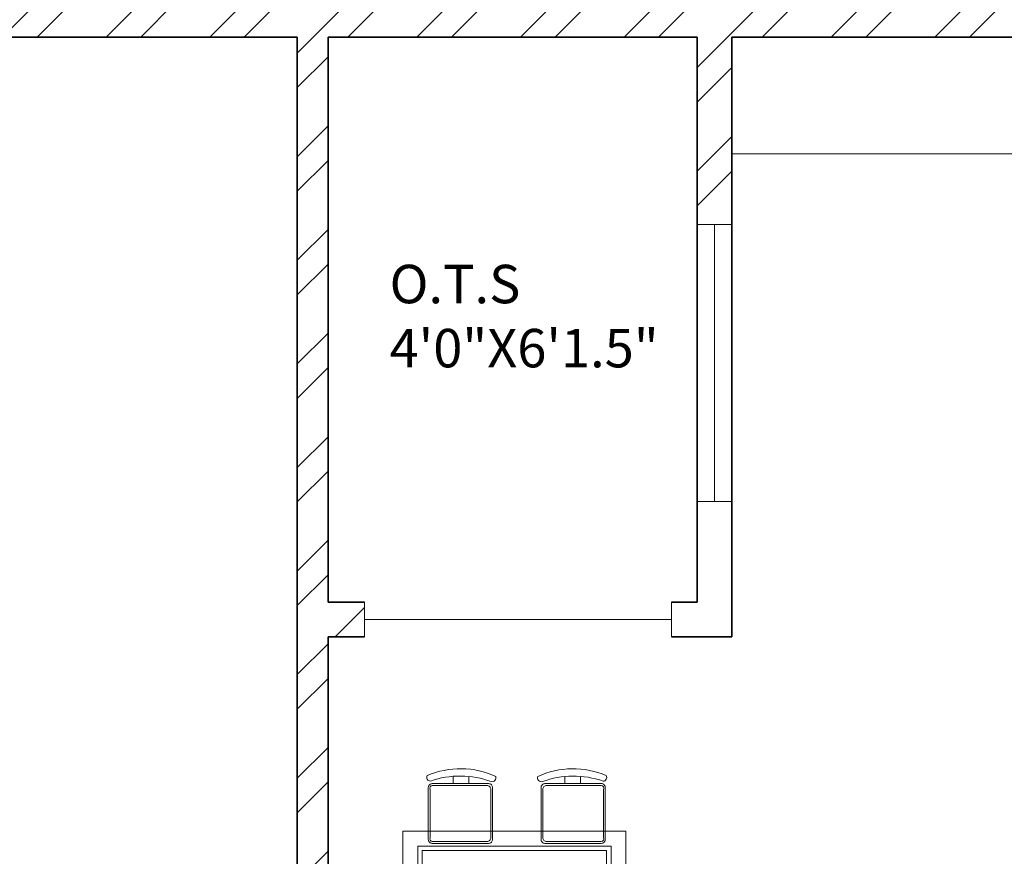
# Model space of a CAD drawing. Units: inches. Extents: x 2120 to 4013, y 1390 to 3019.
# Tile 30 of 59: x 2356 to 2484, y 1964 to 2073. Entities that reach past the tile are written whole.
import ezdxf

# ---------------------------------------------------------------- set-up
doc = ezdxf.new("R2010")
doc.units = ezdxf.units.IN
for name, color, linetype, lineweight in [('A-AREA-IDEN', 7, 'Continuous', 18), ('A-FLOR-CASE', 8, 'Continuous', 18), ('A-FURN', 8, 'Continuous', 13), ('A-GLAZ', 4, 'Continuous', 18), ('A-WALL', 7, 'Continuous', 35), ('A-WALL-PATT', 252, 'Continuous', 13)]:
    doc.layers.add(name, color=color, linetype=linetype, lineweight=lineweight)
doc.styles.get("Standard").update_dxf_attribs({"font": 'arial.ttf'})

# ---------------------------------------------------------------- blocks, each defined once
blk = doc.blocks.new('WIN-PLAN-36IN-02')
for p, q in [((2.25, 36), (0, 36)), ((0, 36), (4.5, 36)), ((2.25, 0), (2.25, 36)), ((0, 0), (4.5, 0)), ((4.5, 0), (2.25, 0))]:
    blk.add_line(p, q)
blk = doc.blocks.new('WIN-PLAN-40IN')
for p, q in [((0, 4.5), (0, 0)), ((39.95, 4.5), (39.95, 0)), ((39.95, 2.25), (0, 2.25)), ((39.95, 0), (39.95, 2.25))]:
    blk.add_line(p, q)
blk = doc.blocks.new('TABLE-DINING')
for points in [[(0, 17.41), (29.01, 17.41), (29.01, 0), (0, 0)], [(1.93, 15.47), (27.08, 15.47), (27.08, 1.93), (1.93, 1.93)], [(2.51, 14.89), (26.5, 14.89), (26.5, 2.51), (2.51, 2.51)]]:
    blk.add_lwpolyline(points, close=True)
blk = doc.blocks.new('CHAIR-DINING-01')
for points in [[(1.68, 0.62, -0.578392), (1.02, 0.02, -0.214524), (0.9, 8.94, -0.552014), (1.62, 8.52, 0.175809), (1.68, 0.62)], [(1.93, 8.29, -0.414214), (2.45, 8.81), (9.19, 8.81, -0.414214), (9.7, 8.29), (9.7, 0.96, -0.414214), (9.19, 0.45), (2.45, 0.45, -0.414214), (1.93, 0.96), (1.93, 8.29)], [(1.93, 3.54), (1.01, 3.54, 0.064759)]]:
    blk.add_lwpolyline(points, format="xyb")
blk.add_lwpolyline([(2.16, 8.29), (2.16, 1.19, 0.414214), (2.68, 0.68), (8.96, 0.68, 0.414214), (9.47, 1.19), (9.47, 8.29, 0.512069), (8.96, 8.58), (2.68, 8.58, 0.512069)], format="xyb", close=True)
blk.add_lwpolyline([(0.99, 5.59), (1.93, 5.59)])
blk = doc.blocks.new('CHAIR-DINING-05')
for points in [[(1.68, 0.62, -0.578392), (1.02, 0.02, -0.214524), (0.9, 8.94, -0.552014), (1.62, 8.52, 0.175809), (1.68, 0.62)], [(1.93, 8.29, -0.414214), (2.45, 8.81), (9.19, 8.81, -0.414214), (9.7, 8.29), (9.7, 0.96, -0.414214), (9.19, 0.45), (2.45, 0.45, -0.414214), (1.93, 0.96), (1.93, 8.29)], [(1.93, 3.54), (1.01, 3.54, 0.064759)]]:
    blk.add_lwpolyline(points, format="xyb")
blk.add_lwpolyline([(2.16, 8.29), (2.16, 1.19, 0.414214), (2.68, 0.68), (8.96, 0.68, 0.414214), (9.47, 1.19), (9.47, 8.29, 0.512069), (8.96, 8.58), (2.68, 8.58, 0.512069)], format="xyb", close=True)
blk.add_lwpolyline([(0.99, 5.59), (1.93, 5.59)])
blk = doc.blocks.new('CHAIR-DINING-08')
for points in [[(0.47, 8.09, -0.175809), (8.38, 8.03, 0.578392), (8.97, 8.69, 0.214524), (0.06, 8.81, 0.552014), (0.47, 8.09, -0.065079)], [(8.04, 7.77), (0.71, 7.77, 0.414214), (0.19, 7.26), (0.19, 0.51, 0.414214), (0.71, 0), (8.04, 0, 0.414214), (8.55, 0.51), (8.55, 7.26, 0.414214), (8.04, 7.77)], [(5.46, 7.77), (5.46, 8.7, -0.064759)]]:
    blk.add_lwpolyline(points, format="xyb")
blk.add_lwpolyline([(3.41, 8.72), (3.41, 7.77)])
blk.add_lwpolyline([(0.71, 7.54), (7.81, 7.54, -0.414214), (8.32, 7.03), (8.32, 0.74, -0.414214), (7.81, 0.23), (0.71, 0.23, -0.512069), (0.42, 0.74), (0.42, 7.03, -0.512069)], format="xyb", close=True)
blk = doc.blocks.new('CHAIR-DINING-13')
for points in [[(0.47, 8.09, -0.175809), (8.38, 8.03, 0.578392), (8.97, 8.69, 0.214524), (0.06, 8.81, 0.552014), (0.47, 8.09, -0.065079)], [(8.04, 7.77), (0.71, 7.77, 0.414214), (0.19, 7.26), (0.19, 0.51, 0.414214), (0.71, 0), (8.04, 0, 0.414214), (8.55, 0.51), (8.55, 7.26, 0.414214), (8.04, 7.77)], [(5.46, 7.77), (5.46, 8.7, -0.064759)]]:
    blk.add_lwpolyline(points, format="xyb")
blk.add_lwpolyline([(3.41, 8.72), (3.41, 7.77)])
blk.add_lwpolyline([(0.71, 7.54), (7.81, 7.54, -0.414214), (8.32, 7.03), (8.32, 0.74, -0.414214), (7.81, 0.23), (0.71, 0.23, -0.512069), (0.42, 0.74), (0.42, 7.03, -0.512069)], format="xyb", close=True)

msp = doc.modelspace()

# ---------------------------------------------------------------- hatches: boundary and pattern name
at = {"layer": 'A-WALL-PATT'}
h = msp.add_hatch(dxfattribs=at)
h.set_pattern_fill('ANSI32', color=256)
h.paths.add_polyline_path([(2271.7331, 2343.531), (2283.3788, 2343.531), (2283.3788, 2348.031), (2283.3788, 2352.5306), (2262.7331, 2352.5306), (2262.7331, 2182.638), (2267.2331, 2182.638), (2271.7331, 2182.638), (2271.7331, 2219.031), (2391.7331, 2219.031), (2391.7331, 2214.189), (2393.9831, 2214.189), (2396.2331, 2214.189), (2396.2331, 2219.031), (2420.2331, 2219.031), (2420.2331, 2225.7535), (2417.2197, 2225.7535), (2415.7331, 2225.7535), (2415.7331, 2223.5306), (2271.7331, 2223.5306)])
h.paths.add_polyline_path([(2380.0942, 2352.5306), (2343.3788, 2352.5306), (2343.3788, 2343.531), (2363.2331, 2343.531), (2363.2331, 2288.8489), (2365.4831, 2288.8489), (2367.7331, 2288.8489), (2367.7331, 2343.531), (2380.0942, 2343.531)], flags=17)
h.paths.add_polyline_path([(2432.4339, 2352.5306), (2404.0943, 2352.5306), (2404.0943, 2343.531), (2415.7331, 2343.531), (2415.7331, 2264.0306), (2367.7331, 2264.0306), (2367.7331, 2266.4872), (2363.2331, 2266.4872), (2363.2331, 2259.531), (2367.7331, 2259.531), (2415.7331, 2259.531), (2415.7331, 2255.0658), (2420.2331, 2255.0658), (2420.2331, 2259.531), (2424.5717, 2259.531), (2424.5717, 2261.781), (2424.5717, 2264.0306), (2420.2331, 2264.0306), (2420.2331, 2343.531), (2432.4339, 2343.531)])
h.paths.add_polyline_path([(2508.9115, 2352.5306), (2456.4339, 2352.5306), (2456.4339, 2343.531), (2468.2331, 2343.531), (2468.2331, 2264.0306), (2448.0487, 2264.0306), (2448.0487, 2259.531), (2468.2331, 2259.531), (2468.2331, 2255.5496), (2472.7331, 2255.5496), (2472.7331, 2343.531), (2508.9115, 2343.531)])
h.paths.add_polyline_path([(2637.7331, 2352.5306), (2544.9116, 2352.5306), (2544.9116, 2343.531), (2589.7331, 2343.531), (2633.2331, 2343.531), (2637.7331, 2343.531)])
h.paths.add_polyline_path([(2594.2331, 2343.5306), (2589.7331, 2343.5306), (2589.7331, 2259.5306), (2589.7331, 2252.4915), (2591.9831, 2252.4915), (2594.2331, 2252.4915)])
h.paths.add_polyline_path([(2637.7331, 2223.5306), (2594.2331, 2223.5306), (2594.2331, 2230.1988), (2591.9831, 2230.1988), (2589.7331, 2230.1988), (2589.7331, 2223.5306), (2472.7331, 2223.5306), (2468.2331, 2223.5306), (2468.2331, 2219.031), (2628.7331, 2219.031), (2628.7331, 2138.031), (2637.7331, 2138.031)])
h.paths.add_polyline_path([(3822.6535, 2458.4402), (3874.9468, 2458.4402), (3874.9468, 2476.9866), (3822.6535, 2476.9866)], flags=9)
h.paths.add_polyline_path([(3834.6921, 2781.8174), (3935.9206, 2781.8174), (3935.9206, 2800.3638), (3834.6921, 2800.3638)], flags=9)
h.paths.add_polyline_path([(3832.2843, 2837.9683), (3884.5776, 2837.9683), (3884.5776, 2856.5146), (3832.2843, 2856.5146)], flags=9)
h.paths.add_polyline_path([(3830.9388, 2861.4782), (3956.8958, 2861.4782), (3956.8958, 2880.0245), (3830.9388, 2880.0245)], flags=9)
h.paths.add_polyline_path([(3870.6966, 2352.5752), (3887.9272, 2352.5752), (3887.9272, 2377.3037), (3870.6966, 2377.3037)], flags=9)
h.paths.add_polyline_path([(3289.2701, 2413.161), (3435.2223, 2413.161), (3435.2223, 2450.2538), (3289.2701, 2450.2538)], flags=9)
h.paths.add_polyline_path([(2487.6944, 2414.3601), (2637.8335, 2414.3601), (2637.8335, 2451.4528), (2487.6944, 2451.4528)], flags=9)
h.paths.add_polyline_path([(2567.3724, 1457.9199), (2815.296, 1457.9199), (2815.296, 1495.0127), (2567.3724, 1495.0127)], flags=9)
h.paths.add_polyline_path([(2655.3825, 2093.2363), (2685.9555, 2093.2363), (2685.9555, 2111.8937), (2655.3825, 2111.8937)], flags=9)
h.paths.add_polyline_path([(2543.9218, 1550.6671), (2587.8406, 1550.6671), (2587.8406, 1569.3244), (2543.9218, 1569.3244)], flags=9)
h.paths.add_polyline_path([(2905.1384, 1543.8113), (2949.0572, 1543.8113), (2949.0572, 1562.4686), (2905.1384, 1562.4686)], flags=9)
h.paths.add_polyline_path([(2736.4118, 1702.4736), (2784.2153, 1702.4736), (2784.2153, 1721.1309), (2736.4118, 1721.1309)], flags=9)
h.paths.add_polyline_path([(2912.8666, 1710.4168), (2951.707, 1710.4168), (2951.707, 1729.0741), (2912.8666, 1729.0741)], flags=9)
h.paths.add_polyline_path([(2923.5785, 1763.5038), (2959.7279, 1763.5038), (2959.7279, 1782.1611), (2923.5785, 1782.1611)], flags=9)
h.paths.add_polyline_path([(2925.2114, 1809.6137), (2967.1861, 1809.6137), (2967.1861, 1828.271), (2925.2114, 1828.271)], flags=9)
h.paths.add_polyline_path([(2996.2711, 1878.9003), (2996.2711, 1913.109), (2977.6138, 1913.109), (2977.6138, 1878.9003)], flags=9)
h.paths.add_polyline_path([(2883.0859, 1895.7192), (2927.1855, 1895.7192), (2927.1855, 1914.3766), (2883.0859, 1914.3766)], flags=9)
h.paths.add_polyline_path([(2787.3924, 1810.8013), (2841.0213, 1810.8013), (2841.0213, 1829.4587), (2787.3924, 1829.4587)], flags=9)
h.paths.add_polyline_path([(2775.6399, 2101.7395), (2829.2689, 2101.7395), (2829.2689, 2120.3968), (2775.6399, 2120.3968)], flags=9)
h.paths.add_polyline_path([(2913.0263, 2075.817), (2951.8667, 2075.817), (2951.8667, 2094.4744), (2913.0263, 2094.4744)], flags=9)
h.paths.add_polyline_path([(2929.966, 2133.3669), (2966.1154, 2133.3669), (2966.1154, 2152.0243), (2929.966, 2152.0243)], flags=9)
h.paths.add_polyline_path([(2932.7502, 2182.6088), (2968.8996, 2182.6088), (2968.8996, 2201.2662), (2932.7502, 2201.2662)], flags=9)
h.paths.add_polyline_path([(2996.0681, 2266.3173), (2996.0681, 2300.5261), (2977.4108, 2300.5261), (2977.4108, 2266.3173)], flags=9)
h.paths.add_polyline_path([(2885.1039, 2279.2186), (2929.2035, 2279.2186), (2929.2035, 2297.8759), (2885.1039, 2297.8759)], flags=9)
h.paths.add_polyline_path([(2735.7042, 2218.3197), (2783.5078, 2218.3197), (2783.5078, 2236.9771), (2735.7042, 2236.9771)], flags=9)
h.paths.add_polyline_path([(2635.6049, 2044.0085), (2648.9678, 2044.0085), (2648.9678, 2054.312), (2635.6049, 2054.312)], flags=9)
h.paths.add_polyline_path([(2714.0148, 1923.0473), (2727.3777, 1923.0473), (2727.3777, 1933.3508), (2714.0148, 1933.3508)], flags=9)
h.paths.add_polyline_path([(2709.0345, 1988.1628), (2722.3974, 1988.1628), (2722.3974, 1998.4663), (2709.0345, 1998.4663)], flags=9)
h.paths.add_polyline_path([(2592.8935, 1962.1763), (2606.2564, 1962.1763), (2606.2564, 1972.4799), (2592.8935, 1972.4799)], flags=9)
h.paths.add_polyline_path([(2618.3996, 1985.9724), (2644.1942, 1985.9724), (2644.1942, 1996.2759), (2618.3996, 1996.2759)], flags=9)
h.paths.add_polyline_path([(2601.279, 1920.5869), (2614.6419, 1920.5869), (2614.6419, 1930.8904), (2601.279, 1930.8904)], flags=9)
h.paths.add_polyline_path([(2692.3278, 1932.7645), (2704.5311, 1932.7645), (2704.5311, 1943.0681), (2692.3278, 1943.0681)], flags=9)
h.paths.add_polyline_path([(2311.122, 1672.7318), (2355.0408, 1672.7318), (2355.0408, 1691.3892), (2311.122, 1691.3892)], flags=9)
h.paths.add_polyline_path([(2456.2551, 1632.3198), (2492.4796, 1632.3198), (2492.4796, 1650.9772), (2456.2551, 1650.9772)], flags=9)
h.paths.add_polyline_path([(2401.0766, 1631.4793), (2437.301, 1631.4793), (2437.301, 1650.1367), (2401.0766, 1650.1367)], flags=9)
h.paths.add_polyline_path([(2546.7054, 1700.9235), (2594.509, 1700.9235), (2594.509, 1719.5809), (2546.7054, 1719.5809)], flags=9)
h.paths.add_polyline_path([(2445.4866, 1766.9937), (2497.5261, 1766.9937), (2497.5261, 1785.651), (2445.4866, 1785.651)], flags=9)
h.paths.add_polyline_path([(2287.9992, 1739.7675), (2326.8396, 1739.7675), (2326.8396, 1758.4248), (2287.9992, 1758.4248)], flags=9)
h.paths.add_polyline_path([(2458.5279, 1924.7607), (2510.5675, 1924.7607), (2510.5675, 1943.4181), (2458.5279, 1943.4181)], flags=9)
h.paths.add_polyline_path([(2309.2811, 1902.7642), (2345.4305, 1902.7642), (2345.4305, 1921.4215), (2309.2811, 1921.4215)], flags=9)
h.paths.add_polyline_path([(2490.7554, 2018.9392), (2530.7896, 2018.9392), (2530.7896, 2037.5965), (2490.7554, 2037.5965)], flags=9)
h.paths.add_polyline_path([(2402.143, 2024.7393), (2438.5414, 2024.7393), (2438.5414, 2043.3966), (2402.143, 2043.3966)], flags=9)
h.paths.add_polyline_path([(2287.856, 1931.7926), (2326.6964, 1931.7926), (2326.6964, 1950.4499), (2287.856, 1950.4499)], flags=9)
h.paths.add_polyline_path([(2281.7979, 2193.5771), (2320.6383, 2193.5771), (2320.6383, 2212.2344), (2281.7979, 2212.2344)], flags=25)
h.paths.add_polyline_path([(2484.0754, 2093.892), (2536.115, 2093.892), (2536.115, 2112.5494), (2484.0754, 2112.5494)], flags=9)
h.paths.add_polyline_path([(2624.7948, 2281.8639), (2624.7948, 2311.4137), (2606.1375, 2311.4137), (2606.1375, 2281.8639)], flags=9)
h.paths.add_polyline_path([(2507.5036, 2290.3639), (2541.934, 2290.3639), (2541.934, 2309.0212), (2507.5036, 2309.0212)], flags=9)
h.paths.add_polyline_path([(2423.1076, 2285.2202), (2459.332, 2285.2202), (2459.332, 2303.8776), (2423.1076, 2303.8776)], flags=9)
h.paths.add_polyline_path([(2374.5467, 2289.6272), (2410.7711, 2289.6272), (2410.7711, 2308.2846), (2374.5467, 2308.2846)], flags=25)
h.paths.add_polyline_path([(2277.4907, 2227.5651), (2316.3311, 2227.5651), (2316.3311, 2246.2224), (2277.4907, 2246.2224)], flags=25)
h.paths.add_polyline_path([(2655.3825, 2093.2367), (2685.9555, 2093.2367), (2685.9555, 2111.894), (2655.3825, 2111.894)], flags=9)
h.paths.add_polyline_path([(2543.9217, 1550.6674), (2587.8406, 1550.6674), (2587.8406, 1569.3247), (2543.9217, 1569.3247)], flags=9)
h.paths.add_polyline_path([(2905.1384, 1543.8116), (2949.0572, 1543.8116), (2949.0572, 1562.4689), (2905.1384, 1562.4689)], flags=9)
h.paths.add_polyline_path([(2736.4118, 1702.4739), (2784.2153, 1702.4739), (2784.2153, 1721.1312), (2736.4118, 1721.1312)], flags=9)
h.paths.add_polyline_path([(2912.8666, 1710.4171), (2951.707, 1710.4171), (2951.707, 1729.0744), (2912.8666, 1729.0744)], flags=9)
h.paths.add_polyline_path([(2923.5785, 1763.5041), (2959.7279, 1763.5041), (2959.7279, 1782.1614), (2923.5785, 1782.1614)], flags=9)
h.paths.add_polyline_path([(2925.2114, 1809.614), (2967.1861, 1809.614), (2967.1861, 1828.2713), (2925.2114, 1828.2713)], flags=9)
h.paths.add_polyline_path([(2996.2711, 1878.9006), (2996.2711, 1913.1094), (2977.6137, 1913.1094), (2977.6137, 1878.9006)], flags=9)
h.paths.add_polyline_path([(2883.0859, 1895.7195), (2927.1855, 1895.7195), (2927.1855, 1914.3769), (2883.0859, 1914.3769)], flags=9)
h.paths.add_polyline_path([(2787.3924, 1810.8016), (2841.0213, 1810.8016), (2841.0213, 1829.459), (2787.3924, 1829.459)], flags=9)
h.paths.add_polyline_path([(2775.6399, 2101.7398), (2829.2688, 2101.7398), (2829.2688, 2120.3971), (2775.6399, 2120.3971)], flags=9)
h.paths.add_polyline_path([(2913.0263, 2075.8173), (2951.8667, 2075.8173), (2951.8667, 2094.4747), (2913.0263, 2094.4747)], flags=9)
h.paths.add_polyline_path([(2929.966, 2133.3672), (2966.1154, 2133.3672), (2966.1154, 2152.0246), (2929.966, 2152.0246)], flags=9)
h.paths.add_polyline_path([(2932.7502, 2182.6091), (2968.8996, 2182.6091), (2968.8996, 2201.2665), (2932.7502, 2201.2665)], flags=9)
h.paths.add_polyline_path([(2996.0681, 2266.3176), (2996.0681, 2300.5264), (2977.4108, 2300.5264), (2977.4108, 2266.3176)], flags=9)
h.paths.add_polyline_path([(2885.1039, 2279.2189), (2929.2035, 2279.2189), (2929.2035, 2297.8762), (2885.1039, 2297.8762)], flags=9)
h.paths.add_polyline_path([(2735.7042, 2218.32), (2783.5078, 2218.32), (2783.5078, 2236.9774), (2735.7042, 2236.9774)], flags=9)
h.paths.add_polyline_path([(2635.6048, 2044.0088), (2648.9677, 2044.0088), (2648.9677, 2054.3123), (2635.6048, 2054.3123)], flags=9)
h.paths.add_polyline_path([(2714.0148, 1923.0476), (2727.3777, 1923.0476), (2727.3777, 1933.3511), (2714.0148, 1933.3511)], flags=9)
h.paths.add_polyline_path([(2709.0345, 1988.1631), (2722.3974, 1988.1631), (2722.3974, 1998.4666), (2709.0345, 1998.4666)], flags=9)
h.paths.add_polyline_path([(2592.8935, 1962.1766), (2606.2564, 1962.1766), (2606.2564, 1972.4802), (2592.8935, 1972.4802)], flags=9)
h.paths.add_polyline_path([(2618.3995, 1985.9727), (2644.1942, 1985.9727), (2644.1942, 1996.2762), (2618.3995, 1996.2762)], flags=9)
h.paths.add_polyline_path([(2601.279, 1920.5872), (2614.6419, 1920.5872), (2614.6419, 1930.8908), (2601.279, 1930.8908)], flags=9)
h.paths.add_polyline_path([(2692.3278, 1932.7648), (2704.5311, 1932.7648), (2704.5311, 1943.0684), (2692.3278, 1943.0684)], flags=9)
h.paths.add_polyline_path([(2311.122, 1672.7321), (2355.0408, 1672.7321), (2355.0408, 1691.3895), (2311.122, 1691.3895)], flags=9)
h.paths.add_polyline_path([(2456.2551, 1632.3201), (2492.4795, 1632.3201), (2492.4795, 1650.9775), (2456.2551, 1650.9775)], flags=9)
h.paths.add_polyline_path([(2401.0766, 1631.4796), (2437.301, 1631.4796), (2437.301, 1650.137), (2401.0766, 1650.137)], flags=9)
h.paths.add_polyline_path([(2546.7054, 1700.9238), (2594.509, 1700.9238), (2594.509, 1719.5812), (2546.7054, 1719.5812)], flags=9)
h.paths.add_polyline_path([(2445.4866, 1766.994), (2497.5261, 1766.994), (2497.5261, 1785.6513), (2445.4866, 1785.6513)], flags=9)
h.paths.add_polyline_path([(2287.9992, 1739.7678), (2326.8396, 1739.7678), (2326.8396, 1758.4251), (2287.9992, 1758.4251)], flags=9)
h.paths.add_polyline_path([(2458.5279, 1924.7611), (2510.5675, 1924.7611), (2510.5675, 1943.4184), (2458.5279, 1943.4184)], flags=9)
h.paths.add_polyline_path([(2309.2811, 1902.7645), (2345.4305, 1902.7645), (2345.4305, 1921.4218), (2309.2811, 1921.4218)], flags=9)
h.paths.add_polyline_path([(2490.7554, 2018.9395), (2530.7895, 2018.9395), (2530.7895, 2037.5968), (2490.7554, 2037.5968)], flags=9)
h.paths.add_polyline_path([(2402.143, 2024.7396), (2438.5413, 2024.7396), (2438.5413, 2043.3969), (2402.143, 2043.3969)], flags=9)
h.paths.add_polyline_path([(2287.856, 1931.7929), (2326.6964, 1931.7929), (2326.6964, 1950.4502), (2287.856, 1950.4502)], flags=9)
h.paths.add_polyline_path([(2281.7979, 2193.5774), (2320.6383, 2193.5774), (2320.6383, 2212.2347), (2281.7979, 2212.2347)], flags=25)
h.paths.add_polyline_path([(2484.0754, 2093.8924), (2536.115, 2093.8924), (2536.115, 2112.5497), (2484.0754, 2112.5497)], flags=9)
h.paths.add_polyline_path([(2624.7948, 2281.8642), (2624.7948, 2311.414), (2606.1374, 2311.414), (2606.1374, 2281.8642)], flags=9)
h.paths.add_polyline_path([(2507.5035, 2290.3642), (2541.934, 2290.3642), (2541.934, 2309.0215), (2507.5035, 2309.0215)], flags=9)
h.paths.add_polyline_path([(2423.1075, 2285.2205), (2459.332, 2285.2205), (2459.332, 2303.8779), (2423.1075, 2303.8779)], flags=9)
h.paths.add_polyline_path([(2374.5467, 2289.6275), (2410.7711, 2289.6275), (2410.7711, 2308.2849), (2374.5467, 2308.2849)], flags=25)
h.paths.add_polyline_path([(2277.4907, 2227.5654), (2316.3311, 2227.5654), (2316.3311, 2246.2227), (2277.4907, 2246.2227)], flags=25)
h = msp.add_hatch(dxfattribs=at)
h.set_pattern_fill('ANSI32', color=256)
h.paths.add_polyline_path([(2271.7331, 1980.389), (2262.7331, 1980.389), (2262.7331, 1912.8434), (2267.2331, 1912.8434), (2271.7331, 1912.8434), (2271.7331, 1922.531), (2351.2331, 1922.531), (2351.2331, 1901.4728), (2355.7331, 1901.4728), (2355.7331, 1922.531), (2357.9815, 1922.531), (2357.9815, 1926.5306), (2271.7331, 1926.5306)])
h.paths.add_polyline_path([(2589.2331, 1949.1622), (2584.7331, 1949.1622), (2580.2331, 1949.1622), (2580.2331, 1874.5306), (2355.7331, 1874.5306), (2355.7331, 1880.1922), (2351.2331, 1880.1922), (2351.2331, 1874.5306), (2271.7331, 1874.5306), (2271.7331, 1888.8431), (2262.7331, 1888.8431), (2262.7331, 1842.2909), (2267.2331, 1842.2909), (2271.7331, 1842.2909), (2271.7331, 1865.531), (2415.7331, 1865.531), (2415.7331, 1779.7286), (2420.2331, 1779.7286), (2420.2331, 1865.531), (2589.2331, 1865.531)])
h.paths.add_polyline_path([(2271.7331, 1782.2906), (2262.7331, 1782.2906), (2262.7331, 1711.4639), (2267.2331, 1711.4639), (2271.7331, 1711.4639), (2271.7331, 1738.031), (2420.2331, 1738.031), (2420.2331, 1742.531), (2420.2331, 1747.3376), (2417.9831, 1747.3376), (2415.7331, 1747.3376), (2415.7331, 1742.5306), (2271.7331, 1742.5306)])
h.paths.add_polyline_path([(2271.7331, 1627.031), (2362.3957, 1627.031), (2362.3957, 1629.281), (2362.3957, 1631.5306), (2271.7331, 1631.5306), (2271.7331, 1675.4636), (2262.7331, 1675.4636), (2262.7331, 1581.531), (2405.3032, 1581.531), (2405.3032, 1586.031), (2405.3032, 1590.5306), (2396.2331, 1590.5306), (2396.2331, 1691.4513), (2418.7206, 1691.4513), (2418.7206, 1695.951), (2396.2331, 1695.951), (2391.7331, 1695.951), (2391.7331, 1631.5306), (2386.7425, 1631.5306), (2386.7425, 1629.2806), (2386.7425, 1627.031), (2391.7331, 1627.031), (2391.7331, 1586.1709), (2271.7331, 1586.1709)])
h.paths.add_polyline_path([(2459.6703, 1590.5306), (2429.3032, 1590.5306), (2429.3032, 1581.531), (2459.6703, 1581.531), (2459.6703, 1586.031)])
h.paths.add_polyline_path([(2501.2331, 1590.531), (2501.2331, 1665.0195), (2498.9831, 1665.0195), (2496.7331, 1665.0195), (2496.7331, 1590.5306), (2483.8201, 1590.5306), (2483.8201, 1590.1579), (2483.6704, 1590.1579), (2483.6704, 1581.531), (2505.0196, 1581.531), (2505.0196, 1583.781), (2505.0196, 1586.0306), (2501.2331, 1586.0306)])
h.paths.add_polyline_path([(2544.1361, 1583.781), (2544.1361, 1586.0306), (2527.1368, 1586.0306), (2527.1368, 1583.7806), (2527.1368, 1581.531), (2544.1361, 1581.531)])
h.paths.add_polyline_path([(3822.6535, 2458.4402), (3874.9468, 2458.4402), (3874.9468, 2476.9866), (3822.6535, 2476.9866)], flags=9)
h.paths.add_polyline_path([(3834.6921, 2781.8174), (3935.9206, 2781.8174), (3935.9206, 2800.3638), (3834.6921, 2800.3638)], flags=9)
h.paths.add_polyline_path([(3832.2843, 2837.9683), (3884.5776, 2837.9683), (3884.5776, 2856.5146), (3832.2843, 2856.5146)], flags=9)
h.paths.add_polyline_path([(3830.9388, 2861.4782), (3956.8958, 2861.4782), (3956.8958, 2880.0245), (3830.9388, 2880.0245)], flags=9)
h.paths.add_polyline_path([(3870.6966, 2352.5752), (3887.9272, 2352.5752), (3887.9272, 2377.3037), (3870.6966, 2377.3037)], flags=9)
h.paths.add_polyline_path([(3289.2701, 2413.161), (3435.2223, 2413.161), (3435.2223, 2450.2538), (3289.2701, 2450.2538)], flags=9)
h.paths.add_polyline_path([(2487.6944, 2414.3601), (2637.8335, 2414.3601), (2637.8335, 2451.4528), (2487.6944, 2451.4528)], flags=9)
h.paths.add_polyline_path([(2567.3724, 1457.9199), (2815.296, 1457.9199), (2815.296, 1495.0127), (2567.3724, 1495.0127)], flags=9)
h.paths.add_polyline_path([(2655.3825, 2093.2363), (2685.9555, 2093.2363), (2685.9555, 2111.8937), (2655.3825, 2111.8937)], flags=9)
h.paths.add_polyline_path([(2543.9218, 1550.6671), (2587.8406, 1550.6671), (2587.8406, 1569.3244), (2543.9218, 1569.3244)], flags=9)
h.paths.add_polyline_path([(2905.1384, 1543.8113), (2949.0572, 1543.8113), (2949.0572, 1562.4686), (2905.1384, 1562.4686)], flags=9)
h.paths.add_polyline_path([(2736.4118, 1702.4736), (2784.2153, 1702.4736), (2784.2153, 1721.1309), (2736.4118, 1721.1309)], flags=9)
h.paths.add_polyline_path([(2912.8666, 1710.4168), (2951.707, 1710.4168), (2951.707, 1729.0741), (2912.8666, 1729.0741)], flags=9)
h.paths.add_polyline_path([(2923.5785, 1763.5038), (2959.7279, 1763.5038), (2959.7279, 1782.1611), (2923.5785, 1782.1611)], flags=9)
h.paths.add_polyline_path([(2925.2114, 1809.6137), (2967.1861, 1809.6137), (2967.1861, 1828.271), (2925.2114, 1828.271)], flags=9)
h.paths.add_polyline_path([(2996.2711, 1878.9003), (2996.2711, 1913.109), (2977.6138, 1913.109), (2977.6138, 1878.9003)], flags=9)
h.paths.add_polyline_path([(2883.0859, 1895.7192), (2927.1855, 1895.7192), (2927.1855, 1914.3766), (2883.0859, 1914.3766)], flags=9)
h.paths.add_polyline_path([(2787.3924, 1810.8013), (2841.0213, 1810.8013), (2841.0213, 1829.4587), (2787.3924, 1829.4587)], flags=9)
h.paths.add_polyline_path([(2775.6399, 2101.7395), (2829.2689, 2101.7395), (2829.2689, 2120.3968), (2775.6399, 2120.3968)], flags=9)
h.paths.add_polyline_path([(2913.0263, 2075.817), (2951.8667, 2075.817), (2951.8667, 2094.4744), (2913.0263, 2094.4744)], flags=9)
h.paths.add_polyline_path([(2929.966, 2133.3669), (2966.1154, 2133.3669), (2966.1154, 2152.0243), (2929.966, 2152.0243)], flags=9)
h.paths.add_polyline_path([(2932.7502, 2182.6088), (2968.8996, 2182.6088), (2968.8996, 2201.2662), (2932.7502, 2201.2662)], flags=9)
h.paths.add_polyline_path([(2996.0681, 2266.3173), (2996.0681, 2300.5261), (2977.4108, 2300.5261), (2977.4108, 2266.3173)], flags=9)
h.paths.add_polyline_path([(2885.1039, 2279.2186), (2929.2035, 2279.2186), (2929.2035, 2297.8759), (2885.1039, 2297.8759)], flags=9)
h.paths.add_polyline_path([(2735.7042, 2218.3197), (2783.5078, 2218.3197), (2783.5078, 2236.9771), (2735.7042, 2236.9771)], flags=9)
h.paths.add_polyline_path([(2635.6049, 2044.0085), (2648.9678, 2044.0085), (2648.9678, 2054.312), (2635.6049, 2054.312)], flags=9)
h.paths.add_polyline_path([(2714.0148, 1923.0473), (2727.3777, 1923.0473), (2727.3777, 1933.3508), (2714.0148, 1933.3508)], flags=9)
h.paths.add_polyline_path([(2709.0345, 1988.1628), (2722.3974, 1988.1628), (2722.3974, 1998.4663), (2709.0345, 1998.4663)], flags=9)
h.paths.add_polyline_path([(2592.8935, 1962.1763), (2606.2564, 1962.1763), (2606.2564, 1972.4799), (2592.8935, 1972.4799)], flags=9)
h.paths.add_polyline_path([(2618.3996, 1985.9724), (2644.1942, 1985.9724), (2644.1942, 1996.2759), (2618.3996, 1996.2759)], flags=9)
h.paths.add_polyline_path([(2601.279, 1920.5869), (2614.6419, 1920.5869), (2614.6419, 1930.8904), (2601.279, 1930.8904)], flags=9)
h.paths.add_polyline_path([(2692.3278, 1932.7645), (2704.5311, 1932.7645), (2704.5311, 1943.0681), (2692.3278, 1943.0681)], flags=9)
h.paths.add_polyline_path([(2311.122, 1672.7318), (2355.0408, 1672.7318), (2355.0408, 1691.3892), (2311.122, 1691.3892)], flags=25)
h.paths.add_polyline_path([(2456.2551, 1632.3198), (2492.4796, 1632.3198), (2492.4796, 1650.9772), (2456.2551, 1650.9772)], flags=9)
h.paths.add_polyline_path([(2401.0766, 1631.4793), (2437.301, 1631.4793), (2437.301, 1650.1367), (2401.0766, 1650.1367)], flags=9)
h.paths.add_polyline_path([(2546.7054, 1700.9235), (2594.509, 1700.9235), (2594.509, 1719.5809), (2546.7054, 1719.5809)], flags=9)
h.paths.add_polyline_path([(2445.4866, 1766.9937), (2497.5261, 1766.9937), (2497.5261, 1785.651), (2445.4866, 1785.651)], flags=9)
h.paths.add_polyline_path([(2287.9992, 1739.7675), (2326.8396, 1739.7675), (2326.8396, 1758.4248), (2287.9992, 1758.4248)], flags=24)
h.paths.add_polyline_path([(2458.5279, 1924.7607), (2510.5675, 1924.7607), (2510.5675, 1943.4181), (2458.5279, 1943.4181)], flags=25)
h.paths.add_polyline_path([(2309.2811, 1902.7642), (2345.4305, 1902.7642), (2345.4305, 1921.4215), (2309.2811, 1921.4215)], flags=25)
h.paths.add_polyline_path([(2490.7554, 2018.9392), (2530.7896, 2018.9392), (2530.7896, 2037.5965), (2490.7554, 2037.5965)], flags=9)
h.paths.add_polyline_path([(2402.143, 2024.7393), (2438.5414, 2024.7393), (2438.5414, 2043.3966), (2402.143, 2043.3966)], flags=9)
h.paths.add_polyline_path([(2287.856, 1931.7926), (2326.6964, 1931.7926), (2326.6964, 1950.4499), (2287.856, 1950.4499)], flags=25)
h.paths.add_polyline_path([(2281.7979, 2193.5771), (2320.6383, 2193.5771), (2320.6383, 2212.2344), (2281.7979, 2212.2344)], flags=9)
h.paths.add_polyline_path([(2484.0754, 2093.892), (2536.115, 2093.892), (2536.115, 2112.5494), (2484.0754, 2112.5494)], flags=9)
h.paths.add_polyline_path([(2624.7948, 2281.8639), (2624.7948, 2311.4137), (2606.1375, 2311.4137), (2606.1375, 2281.8639)], flags=9)
h.paths.add_polyline_path([(2507.5036, 2290.3639), (2541.934, 2290.3639), (2541.934, 2309.0212), (2507.5036, 2309.0212)], flags=9)
h.paths.add_polyline_path([(2423.1076, 2285.2202), (2459.332, 2285.2202), (2459.332, 2303.8776), (2423.1076, 2303.8776)], flags=9)
h.paths.add_polyline_path([(2374.5467, 2289.6272), (2410.7711, 2289.6272), (2410.7711, 2308.2846), (2374.5467, 2308.2846)], flags=9)
h.paths.add_polyline_path([(2277.4907, 2227.5651), (2316.3311, 2227.5651), (2316.3311, 2246.2224), (2277.4907, 2246.2224)], flags=9)
h.paths.add_polyline_path([(2655.3825, 2093.2367), (2685.9555, 2093.2367), (2685.9555, 2111.894), (2655.3825, 2111.894)], flags=9)
h.paths.add_polyline_path([(2543.9217, 1550.6674), (2587.8406, 1550.6674), (2587.8406, 1569.3247), (2543.9217, 1569.3247)], flags=9)
h.paths.add_polyline_path([(2905.1384, 1543.8116), (2949.0572, 1543.8116), (2949.0572, 1562.4689), (2905.1384, 1562.4689)], flags=9)
h.paths.add_polyline_path([(2736.4118, 1702.4739), (2784.2153, 1702.4739), (2784.2153, 1721.1312), (2736.4118, 1721.1312)], flags=9)
h.paths.add_polyline_path([(2912.8666, 1710.4171), (2951.707, 1710.4171), (2951.707, 1729.0744), (2912.8666, 1729.0744)], flags=9)
h.paths.add_polyline_path([(2923.5785, 1763.5041), (2959.7279, 1763.5041), (2959.7279, 1782.1614), (2923.5785, 1782.1614)], flags=9)
h.paths.add_polyline_path([(2925.2114, 1809.614), (2967.1861, 1809.614), (2967.1861, 1828.2713), (2925.2114, 1828.2713)], flags=9)
h.paths.add_polyline_path([(2996.2711, 1878.9006), (2996.2711, 1913.1094), (2977.6137, 1913.1094), (2977.6137, 1878.9006)], flags=9)
h.paths.add_polyline_path([(2883.0859, 1895.7195), (2927.1855, 1895.7195), (2927.1855, 1914.3769), (2883.0859, 1914.3769)], flags=9)
h.paths.add_polyline_path([(2787.3924, 1810.8016), (2841.0213, 1810.8016), (2841.0213, 1829.459), (2787.3924, 1829.459)], flags=9)
h.paths.add_polyline_path([(2775.6399, 2101.7398), (2829.2688, 2101.7398), (2829.2688, 2120.3971), (2775.6399, 2120.3971)], flags=9)
h.paths.add_polyline_path([(2913.0263, 2075.8173), (2951.8667, 2075.8173), (2951.8667, 2094.4747), (2913.0263, 2094.4747)], flags=9)
h.paths.add_polyline_path([(2929.966, 2133.3672), (2966.1154, 2133.3672), (2966.1154, 2152.0246), (2929.966, 2152.0246)], flags=9)
h.paths.add_polyline_path([(2932.7502, 2182.6091), (2968.8996, 2182.6091), (2968.8996, 2201.2665), (2932.7502, 2201.2665)], flags=9)
h.paths.add_polyline_path([(2996.0681, 2266.3176), (2996.0681, 2300.5264), (2977.4108, 2300.5264), (2977.4108, 2266.3176)], flags=9)
h.paths.add_polyline_path([(2885.1039, 2279.2189), (2929.2035, 2279.2189), (2929.2035, 2297.8762), (2885.1039, 2297.8762)], flags=9)
h.paths.add_polyline_path([(2735.7042, 2218.32), (2783.5078, 2218.32), (2783.5078, 2236.9774), (2735.7042, 2236.9774)], flags=9)
h.paths.add_polyline_path([(2635.6048, 2044.0088), (2648.9677, 2044.0088), (2648.9677, 2054.3123), (2635.6048, 2054.3123)], flags=9)
h.paths.add_polyline_path([(2714.0148, 1923.0476), (2727.3777, 1923.0476), (2727.3777, 1933.3511), (2714.0148, 1933.3511)], flags=9)
h.paths.add_polyline_path([(2709.0345, 1988.1631), (2722.3974, 1988.1631), (2722.3974, 1998.4666), (2709.0345, 1998.4666)], flags=9)
h.paths.add_polyline_path([(2592.8935, 1962.1766), (2606.2564, 1962.1766), (2606.2564, 1972.4802), (2592.8935, 1972.4802)], flags=9)
h.paths.add_polyline_path([(2618.3995, 1985.9727), (2644.1942, 1985.9727), (2644.1942, 1996.2762), (2618.3995, 1996.2762)], flags=9)
h.paths.add_polyline_path([(2601.279, 1920.5872), (2614.6419, 1920.5872), (2614.6419, 1930.8908), (2601.279, 1930.8908)], flags=9)
h.paths.add_polyline_path([(2692.3278, 1932.7648), (2704.5311, 1932.7648), (2704.5311, 1943.0684), (2692.3278, 1943.0684)], flags=9)
h.paths.add_polyline_path([(2311.122, 1672.7321), (2355.0408, 1672.7321), (2355.0408, 1691.3895), (2311.122, 1691.3895)], flags=25)
h.paths.add_polyline_path([(2456.2551, 1632.3201), (2492.4795, 1632.3201), (2492.4795, 1650.9775), (2456.2551, 1650.9775)], flags=9)
h.paths.add_polyline_path([(2401.0766, 1631.4796), (2437.301, 1631.4796), (2437.301, 1650.137), (2401.0766, 1650.137)], flags=9)
h.paths.add_polyline_path([(2546.7054, 1700.9238), (2594.509, 1700.9238), (2594.509, 1719.5812), (2546.7054, 1719.5812)], flags=9)
h.paths.add_polyline_path([(2445.4866, 1766.994), (2497.5261, 1766.994), (2497.5261, 1785.6513), (2445.4866, 1785.6513)], flags=9)
h.paths.add_polyline_path([(2287.9992, 1739.7678), (2326.8396, 1739.7678), (2326.8396, 1758.4251), (2287.9992, 1758.4251)], flags=24)
h.paths.add_polyline_path([(2458.5279, 1924.7611), (2510.5675, 1924.7611), (2510.5675, 1943.4184), (2458.5279, 1943.4184)], flags=25)
h.paths.add_polyline_path([(2309.2811, 1902.7645), (2345.4305, 1902.7645), (2345.4305, 1921.4218), (2309.2811, 1921.4218)], flags=25)
h.paths.add_polyline_path([(2490.7554, 2018.9395), (2530.7895, 2018.9395), (2530.7895, 2037.5968), (2490.7554, 2037.5968)], flags=9)
h.paths.add_polyline_path([(2402.143, 2024.7396), (2438.5413, 2024.7396), (2438.5413, 2043.3969), (2402.143, 2043.3969)], flags=9)
h.paths.add_polyline_path([(2287.856, 1931.7929), (2326.6964, 1931.7929), (2326.6964, 1950.4502), (2287.856, 1950.4502)], flags=25)
h.paths.add_polyline_path([(2281.7979, 2193.5774), (2320.6383, 2193.5774), (2320.6383, 2212.2347), (2281.7979, 2212.2347)], flags=9)
h.paths.add_polyline_path([(2484.0754, 2093.8924), (2536.115, 2093.8924), (2536.115, 2112.5497), (2484.0754, 2112.5497)], flags=9)
h.paths.add_polyline_path([(2624.7948, 2281.8642), (2624.7948, 2311.414), (2606.1374, 2311.414), (2606.1374, 2281.8642)], flags=9)
h.paths.add_polyline_path([(2507.5035, 2290.3642), (2541.934, 2290.3642), (2541.934, 2309.0215), (2507.5035, 2309.0215)], flags=9)
h.paths.add_polyline_path([(2423.1075, 2285.2205), (2459.332, 2285.2205), (2459.332, 2303.8779), (2423.1075, 2303.8779)], flags=9)
h.paths.add_polyline_path([(2374.5467, 2289.6275), (2410.7711, 2289.6275), (2410.7711, 2308.2849), (2374.5467, 2308.2849)], flags=9)
h.paths.add_polyline_path([(2277.4907, 2227.5654), (2316.3311, 2227.5654), (2316.3311, 2246.2227), (2277.4907, 2246.2227)], flags=9)
h = msp.add_hatch(dxfattribs=at)
h.set_pattern_fill('ANSI32', color=256)
h.paths.add_polyline_path([(2271.7331, 2122.6377), (2262.7331, 2122.6377), (2262.7331, 2040.3893), (2267.2331, 2040.3893), (2271.7331, 2040.3893), (2271.7331, 2044.8856), (2271.7331, 2070.531), (2391.7331, 2070.531), (2391.7331, 1926.5306), (2388.3993, 1926.5306), (2388.3993, 1922.531), (2395.7331, 1922.531), (2395.7331, 1992.531), (2400.4511, 1992.531), (2400.4511, 1997.0306), (2395.7331, 1997.0306), (2395.7331, 2070.531), (2443.7331, 2070.531), (2443.7331, 2046.1368), (2448.2331, 2046.1368), (2448.2331, 2070.531), (2580.2331, 2070.531), (2580.2331, 1997.0306), (2492.9076, 1997.0306), (2492.9076, 1992.531), (2580.2331, 1992.531), (2580.2331, 1983.9368), (2589.2331, 1983.9368), (2589.2331, 2070.531), (2589.2331, 2075.0306), (2396.2331, 2075.0306), (2396.2331, 2184.3565), (2393.9831, 2184.3565), (2391.7331, 2184.3565), (2391.7331, 2075.0306), (2271.7331, 2075.0306)])
h.paths.add_polyline_path([(2724.7331, 2138.0306), (2628.7331, 2138.0306), (2628.7331, 2070.5306), (2628.7331, 2067.0987), (2633.2331, 2067.0987), (2637.7331, 2067.0987), (2637.7331, 2070.531), (2657.3413, 2070.531), (2657.3413, 2079.5306), (2637.7331, 2079.5306), (2637.7331, 2129.031), (2715.7331, 2129.031), (2715.7331, 2079.5306), (2698.0378, 2079.5306), (2698.0378, 2070.531), (2715.7331, 2070.531), (2715.7331, 2012.1531), (2720.2331, 2012.1531), (2724.7331, 2012.1531)])
h.paths.add_polyline_path([(2724.7331, 2213.031), (2831.3209, 2213.031), (2831.3209, 2215.281), (2831.3209, 2217.5306), (2724.7331, 2217.5306), (2724.7331, 2343.531), (2751.8755, 2343.531), (2751.8755, 2352.5306), (2715.7331, 2352.5306), (2715.7331, 2138.031), (2724.7331, 2138.031)])
h.paths.add_polyline_path([(2902.53, 2352.5306), (2811.8755, 2352.5306), (2811.8755, 2343.531), (2867.2331, 2343.531), (2867.2331, 2217.5306), (2863.6364, 2217.5306), (2863.6364, 2213.031), (2871.7331, 2213.031), (2871.7331, 2217.531), (2871.7331, 2343.531), (2902.53, 2343.531)])
h.paths.add_polyline_path([(3009.7331, 2352.5306), (2938.53, 2352.5306), (2938.53, 2343.531), (2966.2331, 2343.531), (2966.2331, 2242.3281), (2968.4831, 2242.3281), (2970.7331, 2242.3281), (2970.7331, 2343.531), (3009.7331, 2343.531)])
h.paths.add_polyline_path([(3009.7331, 2217.5306), (2970.7331, 2217.5306), (2970.7331, 2220.5422), (2968.4831, 2220.5422), (2966.2331, 2220.5422), (2966.2331, 2217.5306), (2911.7752, 2217.5306), (2907.7331, 2217.5306), (2907.7331, 2213.0306), (2907.7331, 2194.9663), (2912.2331, 2194.9663), (2912.2331, 2213.031), (2970.7331, 2213.031), (3000.7331, 2213.031), (3000.7331, 2205.523), (3009.7331, 2205.523)])
h.paths.add_polyline_path([(3009.7331, 2181.5227), (3000.7331, 2181.5227), (3000.7331, 2165.0306), (2912.2331, 2165.0306), (2912.2331, 2170.8202), (2907.7331, 2170.8202), (2907.7331, 2165.0306), (2899.5169, 2165.0306), (2899.5169, 2162.7806), (2899.5169, 2160.531), (2907.7331, 2160.531), (2907.7331, 2137.3432), (2912.2331, 2137.3432), (2912.2331, 2160.531), (3000.7331, 2160.531), (3000.7331, 2150.4993), (3009.7331, 2150.4993)])
h.paths.add_polyline_path([(3009.7331, 2126.499), (3005.2331, 2126.499), (3000.7331, 2126.499), (3000.7331, 2112.5306), (2912.2331, 2112.5306), (2912.2331, 2115.6036), (2907.7331, 2115.6036), (2907.7331, 2108.031), (3000.7331, 2108.031), (3000.7331, 2084.7256), (3009.7331, 2084.7256)], flags=17)
h.paths.add_polyline_path([(3009.7331, 1971.531), (3009.7331, 2024.7253), (3000.7331, 2024.7253), (3000.7331, 2006.4153), (3000.7331, 1971.5306), (2864.2331, 1971.5306), (2864.2331, 2160.531), (2868.0522, 2160.531), (2868.0522, 2165.0306), (2859.7331, 2165.0306), (2859.7331, 1971.5306), (2724.7331, 1971.5306), (2724.7331, 1977.7012), (2715.7331, 1977.7012), (2715.7331, 1962.5306), (2715.7331, 1950.9035), (2720.2331, 1950.9035), (2724.7331, 1950.9035), (2724.7331, 1962.531), (2855.2331, 1962.531), (2859.7331, 1962.531), (2859.7331, 1835.031), (2864.2331, 1834.8158), (2864.2331, 1962.531), (2958.7331, 1962.531), (2958.7331, 1937.0925), (2963.2331, 1937.0925), (2963.2331, 1962.531), (3000.7331, 1962.531), (3009.7331, 1962.531)])
h.paths.add_polyline_path([(2724.7331, 1728.531), (2822.7164, 1728.531), (2822.7164, 1733.0306), (2724.7331, 1733.0306), (2724.7331, 1779.3416), (2715.7331, 1779.3416), (2715.7331, 1581.531), (2753.02, 1581.531), (2753.02, 1586.031), (2753.02, 1590.5306), (2724.7331, 1590.5306)])
h.paths.add_polyline_path([(2864.2331, 1590.531), (2864.2331, 1787.031), (2868.4075, 1787.031), (2868.4075, 1791.5306), (2859.7331, 1791.5306), (2859.7331, 1739.0306), (2859.7331, 1733.0306), (2854.3125, 1733.0306), (2854.3125, 1728.531), (2859.7331, 1728.531), (2859.7331, 1590.5306), (2813.02, 1590.5306), (2813.02, 1581.531), (2868.4123, 1581.531), (2868.4123, 1583.781), (2868.4123, 1586.0306), (2864.2331, 1586.0306)])
h.paths.add_polyline_path([(3009.7331, 1754.6619), (3000.7331, 1754.6619), (3000.7331, 1739.0306), (2912.2331, 1739.0306), (2912.2331, 1742.2257), (2907.7331, 1742.2257), (2907.7331, 1739.0306), (2907.7331, 1734.531), (3000.7331, 1734.531), (3000.7331, 1590.5306), (3000.7331, 1586.0306), (2971.3921, 1586.0306), (2971.3921, 1581.531), (3009.7331, 1581.531)])
h.paths.add_polyline_path([(2911.3921, 1583.781), (2911.3921, 1586.0306), (2891.2138, 1586.0306), (2891.2138, 1581.531), (2911.3921, 1581.531)])
h.paths.add_polyline_path([(3009.7331, 1799.8422), (3000.7331, 1799.8422), (3000.7331, 1791.5306), (2912.2331, 1791.5306), (2912.2331, 1796.3264), (2909.9831, 1796.3264), (2907.7331, 1796.3264), (2907.7331, 1791.5306), (2902.7033, 1791.5306), (2902.7033, 1787.031), (2907.7331, 1787.031), (2907.7331, 1761.1622), (2912.2331, 1761.1622), (2912.2331, 1787.031), (3000.7331, 1787.031), (3000.7331, 1778.6622), (3009.7331, 1778.6622)])
h.paths.add_polyline_path([(3009.7331, 1839.5306), (2963.2331, 1839.5306), (2963.2331, 1842.8629), (2960.9831, 1842.8629), (2958.7331, 1842.8629), (2958.7331, 1839.5306), (2907.7331, 1839.5306), (2907.7331, 1814.4599), (2912.2331, 1814.4599), (2912.2331, 1835.031), (3000.7331, 1835.031), (3000.7331, 1823.8425), (3009.7331, 1823.8425), (3009.7331, 1835.031)])
h.paths.add_polyline_path([(2963.2331, 1901.0922), (2960.9831, 1901.0922), (2958.7331, 1901.0922), (2958.7331, 1862.8843), (2963.2331, 1862.8843)], flags=17)
h.paths.add_polyline_path([(2724.7331, 1891.9826), (2724.7331, 1914.3416), (2715.7331, 1914.3416), (2715.7331, 1783.8416), (2637.7331, 1783.8416), (2637.7331, 1914.3416), (2628.7331, 1914.3416), (2624.7701, 1914.3416), (2624.7701, 1909.8416), (2624.7701, 1905.3419), (2628.7331, 1905.3419), (2628.7331, 1876.9915), (2628.7331, 1779.3419), (2637.7331, 1779.3419), (2715.7331, 1779.3419), (2724.7331, 1779.3419), (2724.7331, 1835.031)])
h.paths.add_polyline_path([(2637.7331, 1731.531), (2637.7331, 1779.3416), (2628.7331, 1779.3416), (2628.7331, 1731.5306), (2589.2331, 1731.5306), (2535.9814, 1731.5306), (2496.7331, 1731.5306), (2496.7331, 1725.6876), (2498.9831, 1725.6876), (2501.2331, 1725.6876), (2501.2331, 1727.031), (2628.7331, 1727.031), (2628.7331, 1680.4203), (2628.7331, 1590.5306), (2628.7331, 1586.0306), (2604.1361, 1586.0306), (2604.1361, 1581.531), (2637.7331, 1581.531), (2637.7331, 1590.531)])

# ---------------------------------------------------------------- linework, layer by layer
at = {"layer": 'A-FLOR-CASE'}
for p, q in [((2448.2331, 2055.3306), (2560.319, 2055.3306)), ((2448.2331, 2055.3303), (2560.319, 2055.3303))]:
    msp.add_line(p, q, dxfattribs=at)
at = {"layer": 'A-WALL'}
for p, q in [((2271.7331, 2070.531), (2391.7331, 2070.531)), ((2271.7331, 2070.5306), (2391.7331, 2070.5306)), ((2391.7331, 2070.531), (2391.7331, 1926.531)), ((2391.7331, 2070.5306), (2391.7331, 1926.5306)), ((2395.7331, 2070.531), (2395.7331, 1997.031)), ((2395.7331, 2070.531), (2443.7331, 2070.531)), ((2395.7331, 2070.5306), (2443.7331, 2070.5306)), ((2395.7331, 2070.5306), (2395.7331, 1997.0306)), ((2443.7331, 2070.531), (2443.7331, 1997.031)), ((2443.7331, 2070.5306), (2443.7331, 1997.0306)), ((2448.2331, 2070.531), (2448.2331, 1992.531)), ((2448.2331, 2070.531), (2580.2331, 2070.531)), ((2448.2331, 2070.5306), (2580.2331, 2070.5306)), ((2448.2331, 2070.5306), (2448.2331, 1992.5306)), ((2395.7331, 1997.031), (2400.4511, 1997.031)), ((2395.7331, 1997.0306), (2400.4511, 1997.0306)), ((2440.3969, 1997.031), (2443.7331, 1997.031)), ((2440.3969, 1997.0306), (2443.7331, 1997.0306)), ((2395.7331, 1992.531), (2400.4511, 1992.531)), ((2395.7331, 1992.531), (2395.7331, 1922.531)), ((2395.7331, 1992.5306), (2400.4511, 1992.5306)), ((2395.7331, 1992.5306), (2395.7331, 1922.5306)), ((2440.3969, 1992.531), (2448.2331, 1992.531)), ((2440.3969, 1992.5306), (2448.2331, 1992.5306))]:
    msp.add_line(p, q, dxfattribs=at)

# ---------------------------------------------------------------- block references
at = {"layer": 'A-FURN'}
for name, p in [('CHAIR-DINING-13', (2408.5698, 1965.6774)), ('CHAIR-DINING-08', (2408.5698, 1965.6771)), ('TABLE-DINING', (2405.4561, 1949.8472)), ('TABLE-DINING', (2405.4561, 1949.8469))]:
    msp.add_blockref(name, p, dxfattribs=at)
for name, p, rotation in [('CHAIR-DINING-05', (2422.9752, 1975.3819), 269.9999980921791), ('CHAIR-DINING-01', (2422.9752, 1975.3816), 269.9999980921786)]:
    msp.add_blockref(name, p, dxfattribs=dict(at, rotation=rotation))
at = {"layer": 'A-GLAZ', "rotation": 180}
for p in [(2448.2331, 2046.1368), (2448.2331, 2046.1365)]:
    msp.add_blockref('WIN-PLAN-36IN-02', p, dxfattribs=at)
at = {"layer": 'A-GLAZ'}
for p in [(2400.4511, 1992.531), (2400.4511, 1992.5306)]:
    msp.add_blockref('WIN-PLAN-40IN', p, dxfattribs=at)

# ---------------------------------------------------------------- texts
at = {"layer": 'A-AREA-IDEN', "char_height": 5, "attachment_point": 1}
for insert in [(2403.7306, 2040.9123), (2403.7306, 2040.912)]:
    msp.add_mtext_dynamic_manual_height_columns('O.T.S\\P4\'0"X6\'1.5"', width=95.350915, gutter_width=12.5, heights=[0], dxfattribs=dict(at, insert=insert))

doc.saveas('drawing.dxf')
